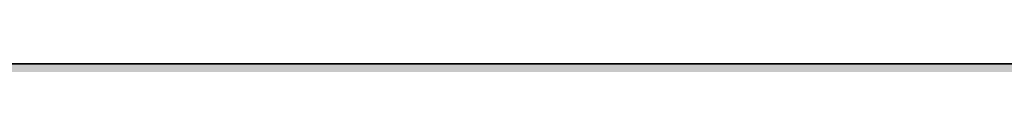
# Model space of a CAD drawing. Units: inches. Extents: x 2091 to 2899, y 967 to 2217.
# Tile 70 of 256: x 2213.35 to 2214.757, y 1099.919 to 1099.919. Entities that reach past the tile are written whole.
import ezdxf

# ---------------------------------------------------------------- set-up
doc = ezdxf.new("R2010")
doc.units = ezdxf.units.IN
doc.layers.add('A-WALL-PATT', color=141, linetype='Continuous', lineweight=13, true_color=0xadddf7)
doc.layers.add('L-SITE-WALL', color=7, linetype='Continuous', lineweight=35)

msp = doc.modelspace()

# ---------------------------------------------------------------- hatches: boundary and pattern name
at = {"layer": 'A-WALL-PATT'}
h = msp.add_hatch(color=256, dxfattribs=at)
h.dxf.hatch_style = 1
h.paths.add_polyline_path([(2212.1436, 1941.4191), (2387.6436, 1941.4191), (2387.6436, 1824.4191), (2392.1436, 1824.4191), (2392.1436, 1941.4191), (2609.6436, 1941.4191), (2609.6436, 1825.9191), (2614.1436, 1825.9191), (2614.1436, 1941.4191), (2794.1436, 1941.4191), (2794.1436, 1928.7622), (2803.1436, 1928.7622), (2803.1436, 2050.9191), (2203.1436, 2050.9191), (2203.1436, 1900.7579), (2212.1436, 1900.7579)])
h.paths.add_polyline_path([(2212.1436, 1945.9191), (2212.1436, 2041.9191), (2794.1436, 2041.9191), (2794.1436, 1945.9191), (2402.2482, 1945.9191), (2401.1024, 1945.7758), (2398.7024, 1945.7758)], flags=16)
h.paths.add_polyline_path([(2230.2299, 1948.0628), (2227.3499, 1949.5028), (2225.9099, 1951.9028), (2223.9899, 1952.8628), (2223.0299, 1955.2628), (2222.0699, 1959.5828), (2222.0699, 1963.4228), (2223.0299, 1965.6628), (2223.9899, 1965.3428), (2225.5859, 1963.8607), (2226.9115, 1964.9573), (2226.9489, 1965.9388), (2227.7783, 1966.9521), (2228.1999, 1968.8787), (2230.7099, 1964.8628), (2233.5899, 1966.3028), (2233.6073, 1966.3319), (2233.7727, 1964.9382), (2234.6338, 1963.6765), (2235.0299, 1963.9028), (2236.282, 1965.5724), (2235.9899, 1962.9428), (2237.9545, 1957.54), (2238.3899, 1957.9028), (2239.2159, 1960.3058), (2238.6546, 1966.385), (2238.6928, 1966.4381), (2238.8406, 1967.4997), (2238.7803, 1967.6875), (2238.8805, 1967.7868), (2238.6669, 1966.2518), (2239.2159, 1960.3058), (2238.3899, 1957.9028), (2236.9499, 1956.7028), (2234.5499, 1949.9828)], flags=0)
h.paths.add_polyline_path([(2278.012, 1948.0628), (2276.4964, 1947.8733), (2275.8498, 1947.6886), (2274.652, 1947.1028)], flags=0)
h.paths.add_polyline_path([(2269.852, 1955.7428), (2268.2762, 1956.6293), (2270.8673, 1956.3484), (2269.372, 1958.1428), (2268.715, 1959.1923), (2270.5698, 1958.7286), (2268.5807, 1961.9061), (2270.812, 1960.8919), (2270.812, 1963.4228), (2271.3933, 1964.7793), (2270.2918, 1966.1562), (2271.772, 1965.6628), (2272.1414, 1966.5248), (2273.9298, 1965.9286), (2275.6304, 1968.0543), (2276.3319, 1966.7219), (2276.5204, 1966.9521), (2276.942, 1968.8787), (2277.7343, 1967.6111), (2278.1399, 1969.4645), (2279.6591, 1967.0337), (2280.412, 1966.7828), (2280.9493, 1967.5888), (2281.6098, 1967.3686), (2282.1333, 1968.1538), (2282.3492, 1966.3334), (2282.3498, 1966.3326), (2283.4076, 1968.0954), (2283.7126, 1965.524), (2284.3202, 1964.6338), (2284.5118, 1964.8892), (2284.235, 1965.7048), (2284.5005, 1967.319), (2284.9079, 1965.4174), (2285.3963, 1966.0686), (2285.4328, 1966.2906), (2285.4733, 1966.1713), (2286.3539, 1967.3454), (2286.222, 1966.1582), (2287.6635, 1968.0802), (2287.714, 1968.4428), (2288.4816, 1969.0167), (2288.574, 1968.7289), (2288.9175, 1969.069), (2288.6068, 1966.8376), (2288.9287, 1963.3513), (2288.935, 1963.3568), (2288.9297, 1963.3404), (2289.0153, 1962.4139), (2290.1112, 1963.8751), (2290.1328, 1963.9426), (2290.2177, 1964.0171), (2290.1112, 1963.8751), (2289.1558, 1960.8916), (2288.594, 1959.2572), (2288.572, 1959.1028), (2289.532, 1960.5428), (2290.012, 1962.4628), (2290.1918, 1962.6427), (2289.7698, 1959.6886), (2286.8898, 1957.2886), (2284.4898, 1950.5686), (2283.3147, 1950.0463), (2283.292, 1949.9828), (2280.2901, 1948.6486), (2281.1298, 1948.6486), (2282.5698, 1948.1686), (2283.2047, 1948.0628), (2278.972, 1948.0628), (2276.092, 1949.5028), (2274.652, 1951.9028), (2272.732, 1952.8628)], flags=0)
h.paths.add_polyline_path([(2271.1589, 1958.0218), (2272.9698, 1955.8486), (2272.0098, 1960.1686), (2272.0098, 1964.0086), (2272.6244, 1965.4427), (2274.328, 1963.8607), (2275.6536, 1964.9573), (2275.6377, 1964.5391), (2277.4122, 1966.0069), (2277.033, 1965.1568), (2276.8299, 1964.9756), (2276.766, 1963.295), (2277.4496, 1962.6602), (2279.452, 1964.8628), (2282.332, 1966.3028), (2283.5298, 1966.8886), (2283.2945, 1966.7709), (2283.913, 1963.8847), (2284.8992, 1964.4483), (2284.732, 1962.9428), (2286.6966, 1957.54), (2287.132, 1957.9028), (2287.5419, 1959.0954), (2287.7794, 1958.4423), (2285.6827, 1956.6951), (2285.8765, 1959.7953), (2284.732, 1962.9428), (2284.8992, 1964.4483), (2283.913, 1963.8847), (2284.2238, 1962.4341), (2283.4244, 1963.6055), (2281.6098, 1962.5686), (2281.1298, 1960.1686), (2282.0898, 1956.3286), (2283.0498, 1952.9686), (2282.5698, 1950.5686), (2280.1698, 1948.6486), (2279.8833, 1948.7919), (2278.972, 1948.0628), (2278.972, 1949.0228), (2278.6723, 1949.3974), (2277.2898, 1950.0886), (2275.8498, 1952.4886), (2273.9298, 1953.4486), (2272.4898, 1954.8886), (2271.9216, 1954.8886), (2271.772, 1955.2628)], flags=0)
h.paths.add_polyline_path([(2311.9941, 1955.7428), (2312.0627, 1955.6742), (2312.0551, 1955.7085)], flags=0)
h.paths.add_polyline_path([(2331.9561, 1963.9518), (2333.3961, 1965.3918), (2331.0771, 1963.3568), (2330.9986, 1963.1115)], flags=0)
h.paths.add_polyline_path([(2310.5541, 1954.3028), (2307.0398, 1956.2799), (2310.7629, 1955.8763), (2312.4741, 1953.8228), (2313.4341, 1951.4228), (2315.3541, 1950.4628), (2316.7941, 1948.0628), (2317.4661, 1947.7268), (2319.3687, 1947.9646), (2317.7541, 1949.9828), (2317.5695, 1950.6105), (2316.7941, 1951.9028), (2314.8741, 1952.8628), (2313.9141, 1955.2628), (2311.5141, 1958.1428), (2309.3755, 1961.5592), (2311.5141, 1960.3371), (2311.5141, 1961.9828), (2310.6047, 1963.1196), (2311.7266, 1962.4785), (2312.4183, 1964.0926), (2312.256, 1964.2955), (2313.1941, 1963.9828), (2313.9141, 1965.6628), (2314.6468, 1965.4186), (2315.3541, 1966.3028), (2316.7941, 1967.7428), (2316.1574, 1966.9469), (2317.0341, 1965.2819), (2317.2226, 1965.5121), (2317.777, 1968.0458), (2318.4741, 1966.7219), (2318.6626, 1966.9521), (2319.0842, 1968.8787), (2321.207, 1965.4821), (2322.1614, 1966.9137), (2322.5541, 1966.7828), (2322.786, 1967.1306), (2322.8816, 1966.3243), (2323.312, 1965.7217), (2323.6513, 1965.8914), (2324.3965, 1967.1334), (2324.6569, 1964.9382), (2324.972, 1964.4766), (2325.3873, 1967.0015), (2325.9408, 1964.4183), (2327.2289, 1966.1358), (2327.1663, 1965.5724), (2328.0591, 1966.7628), (2328.2246, 1966.2475), (2329.668, 1967.6769), (2329.6646, 1967.6875), (2329.7648, 1967.7868), (2329.5511, 1966.2518), (2330.1001, 1960.3058), (2329.3328, 1958.0735), (2329.3131, 1957.9352), (2329.6341, 1958.2028), (2330.2341, 1959.1028), (2330.7141, 1961.0228), (2331.0341, 1961.3428), (2330.7141, 1959.1028), (2329.6341, 1958.2028), (2329.2741, 1957.6628), (2327.7121, 1956.3611), (2325.4341, 1949.9828), (2324.3338, 1949.4937), (2323.9941, 1948.5428), (2319.6741, 1946.6228), (2316.7941, 1948.0628), (2315.3541, 1950.4628), (2313.4341, 1951.4228)], flags=0)
h.paths.add_polyline_path([(2321.3357, 1947.952), (2321.1141, 1948.0628), (2321.1141, 1949.0228), (2319.1941, 1951.4228), (2316.7941, 1959.5828), (2316.6632, 1959.5828), (2315.3541, 1958.1428), (2314.3941, 1958.1428), (2313.1483, 1958.7091), (2312.9541, 1959.5828), (2312.9541, 1960.8919), (2315.8341, 1959.5828), (2316.6632, 1959.5828), (2317.3147, 1960.2994), (2315.0302, 1962.4207), (2316.3558, 1963.5173), (2316.3723, 1963.9516), (2316.4702, 1963.8607), (2317.7958, 1964.9573), (2317.7552, 1963.8897), (2319.1751, 1965.1568), (2319.4984, 1965.8814), (2321.1141, 1965.3428), (2323.2359, 1962.3724), (2325.6863, 1963.7726), (2325.5428, 1962.4806), (2325.1988, 1963.494), (2324.4785, 1963.0824), (2324.926, 1960.9941), (2324.0781, 1962.2365), (2322.4148, 1961.286), (2322.0741, 1959.5828), (2323.0341, 1955.7428), (2323.9941, 1952.3828), (2323.5141, 1949.9828), (2322.1427, 1948.8856), (2322.0741, 1948.5428)], flags=0)
h.paths.add_polyline_path([(2320.2075, 1963.3375), (2320.1541, 1963.4228), (2320.3941, 1963.5428)], flags=0)
h.paths.add_polyline_path([(2353.8505, 1965.8105), (2354.0305, 1965.7505), (2354.3305, 1966.4505), (2354.3305, 1966.9305)], flags=0)
h.paths.add_polyline_path([(2359.0206, 1969.0264), (2359.0984, 1968.9019), (2359.2335, 1969.5195), (2359.2335, 1969.9995)], flags=0)
h.paths.add_polyline_path([(2358.2567, 1966.6817), (2357.9836, 1966.348), (2358.2113, 1966.1462), (2358.4105, 1966.3896)], flags=0)
h.paths.add_polyline_path([(2357.7685, 1966.0588), (2357.7322, 1965.105), (2357.751, 1965.1206), (2357.7695, 1965.6065), (2357.7695, 1966.0578)], flags=0)
h.paths.add_polyline_path([(2359.1115, 1965.3045), (2359.1115, 1964.8245), (2359.8445, 1966.4675), (2359.8445, 1966.9475)], flags=0)
h.paths.add_polyline_path([(2360.2237, 1966.6214), (2360.6985, 1969.3625), (2360.6985, 1969.8425), (2360.2105, 1967.0255), (2360.2105, 1966.6425)], flags=0)
h.paths.add_polyline_path([(2363.4505, 1967.8905), (2363.4505, 1968.3705), (2362.4905, 1966.9305), (2362.656, 1966.6988)], flags=0)
h.paths.add_polyline_path([(2364.4755, 1966.0788), (2365.8505, 1968.3705), (2365.8505, 1968.8505), (2364.428, 1966.4796)], flags=0)
h.paths.add_polyline_path([(2366.3135, 1965.8525), (2366.3667, 1965.6958), (2366.8025, 1968.3455), (2366.8025, 1968.8255)], flags=0)
h.paths.add_polyline_path([(2367.1653, 1965.8035), (2367.2905, 1966.9305), (2367.2905, 1967.4105), (2367.1027, 1965.7201)], flags=0)
h.paths.add_polyline_path([(2370.0365, 1959.9735), (2371.0135, 1963.0245), (2371.0135, 1963.5045), (2370.0365, 1960.4535)], flags=0)
h.paths.add_polyline_path([(2371.6105, 1960.2105), (2372.5705, 1961.6505), (2372.5705, 1962.1305), (2371.8025, 1960.9785)], flags=0)
h.paths.add_polyline_path([(2350.8737, 1956.0051), (2351.9305, 1955.8905), (2354.4905, 1953.3305), (2353.8505, 1954.9305), (2351.4505, 1957.8105), (2347.9355, 1963.4255), (2347.9355, 1963.9055), (2351.4505, 1958.2905), (2353.7051, 1955.585), (2352.8905, 1959.2505), (2352.8905, 1959.7305), (2352.8905, 1961.9248), (2356.7305, 1959.7305), (2358.4545, 1961.6268), (2354.8105, 1965.0105), (2355.0309, 1965.2859), (2358.6911, 1961.8871), (2361.5305, 1965.0105), (2364.3765, 1966.4335), (2364.5244, 1965.1869), (2365.4545, 1963.8242), (2365.8811, 1964.068), (2365.3705, 1966.4505), (2365.3705, 1966.9305), (2366.8105, 1960.2105), (2366.8105, 1959.7305), (2366.3887, 1952.9814), (2367.7705, 1956.8505), (2368.6412, 1957.5761), (2366.8105, 1962.6105), (2366.8105, 1963.0905), (2368.7752, 1957.6877), (2369.2105, 1958.0505), (2370.0016, 1960.3519), (2369.4752, 1966.0527), (2369.5135, 1966.1058), (2369.5142, 1966.1109), (2369.4752, 1966.5327), (2369.5135, 1966.5858), (2369.6146, 1967.3126), (2369.1825, 1968.6585), (2369.1825, 1969.1385), (2369.601, 1967.8352), (2369.7012, 1967.9345), (2369.7179, 1968.0547), (2370.1452, 1968.3741), (2369.7787, 1968.0112), (2369.7012, 1967.4545), (2370.4682, 1968.214), (2369.6749, 1967.2658), (2369.5142, 1966.1109), (2370.0365, 1960.4535), (2370.0365, 1959.9735), (2369.4418, 1958.2432), (2370.6505, 1959.2505), (2371.0458, 1962.0176), (2371.1305, 1962.1305), (2370.6505, 1958.7705), (2367.7705, 1956.3705), (2365.3705, 1949.6505), (2362.0791, 1948.1876), (2363.4505, 1947.7305), (2361.0505, 1947.7305), (2360.0905, 1947.7305), (2357.1039, 1947.3572), (2360.0905, 1948.2105), (2358.1705, 1949.1705), (2356.7305, 1951.5705), (2354.8105, 1952.5305), (2351.9305, 1955.4105)], flags=0)
h.paths.add_polyline_path([(2361.0505, 1948.6905), (2359.1305, 1951.0905), (2356.7305, 1959.2505), (2355.7705, 1959.2505), (2352.8905, 1960.5596), (2352.8905, 1961.4448), (2355.8905, 1959.7305), (2356.7305, 1959.7305), (2356.8372, 1959.3678), (2361.5305, 1964.5305), (2363.2484, 1965.3894), (2364.9253, 1963.0418), (2362.4905, 1961.6505), (2362.0639, 1959.5172), (2362.9705, 1955.8905), (2363.9305, 1952.5305), (2363.9305, 1952.0505), (2363.4505, 1949.6505), (2361.0505, 1947.7305)], flags=0)
h.paths.add_polyline_path([(2359.1305, 1951.5705), (2359.2905, 1951.3705), (2361.0505, 1954.4505), (2361.0505, 1954.9305)], flags=0)
h.paths.add_polyline_path([(2357.2195, 1966.5455), (2356.7925, 1968.8145), (2356.7925, 1969.2945), (2357.2195, 1967.0255)], flags=0)
h.paths.add_polyline_path([(2361.0505, 1954.4505), (2361.5305, 1958.7705), (2361.5305, 1959.2505), (2361.0505, 1954.9305)], flags=0)
h.paths.add_polyline_path([(2402.5483, 1948.4861), (2402.3024, 1948.4158), (2402.5904, 1948.4158)], flags=0)
h.paths.add_polyline_path([(2394.1424, 1956.0958), (2395.6851, 1954.5532), (2396.7205, 1953.9707), (2396.0624, 1955.6158), (2395.2414, 1956.6011), (2395.8789, 1956.4417), (2395.1024, 1959.9358), (2395.1024, 1963.7758), (2396.0624, 1966.0158), (2397.0224, 1965.6958), (2398.6185, 1964.2138), (2399.9441, 1965.3103), (2399.9814, 1966.2918), (2400.8109, 1967.3052), (2401.2325, 1969.2317), (2403.5379, 1965.543), (2403.942, 1967.3893), (2404.7024, 1967.1358), (2405.4603, 1966.0748), (2406.6224, 1966.6558), (2406.6399, 1966.6849), (2406.8052, 1965.2912), (2406.9257, 1965.1147), (2407.3424, 1964.9758), (2407.8743, 1965.7737), (2408.1691, 1964.3981), (2409.3146, 1965.9254), (2409.2175, 1965.0511), (2409.4452, 1963.1312), (2410.3064, 1961.8695), (2410.7024, 1962.0958), (2411.4423, 1963.0823), (2411.1654, 1963.8978), (2411.6164, 1966.6398), (2411.7254, 1966.7911), (2411.8732, 1967.8527), (2411.8129, 1968.0405), (2411.9131, 1968.1398), (2411.6994, 1966.6048), (2412.2484, 1960.6588), (2413.2254, 1963.7098), (2414.3779, 1964.7212), (2414.5132, 1965.6927), (2414.4529, 1965.8805), (2414.5531, 1965.9798), (2414.3779, 1964.7212), (2414.5198, 1964.8457), (2414.3654, 1964.6311), (2414.3394, 1964.4448), (2414.8884, 1958.4988), (2414.0624, 1956.0958), (2412.6224, 1954.8958), (2410.1714, 1948.0329), (2410.0167, 1948.0844), (2405.9024, 1946.2558), (2405.9024, 1947.2158), (2405.2043, 1948.0886), (2404.2224, 1948.4158), (2403.2624, 1948.4158), (2400.3824, 1949.8558), (2399.6624, 1951.0558), (2397.9824, 1952.7358), (2397.0224, 1953.2158), (2395.6851, 1954.5532), (2392.6568, 1956.2569)], flags=0)
h.paths.add_polyline_path([(2409.0857, 1964.4074), (2409.1304, 1964.2757), (2409.2624, 1964.4958)], flags=0)
h.paths.add_polyline_path([(2397.7424, 1961.6158), (2398.7024, 1963.8558), (2399.6624, 1963.5358), (2401.4266, 1965.741), (2401.7914, 1966.5588), (2402.0714, 1965.0708), (2402.8355, 1964.3934), (2403.2624, 1964.9149), (2403.3381, 1964.7711), (2402.6155, 1963.9762), (2402.4986, 1960.9022), (2403.543, 1959.9325), (2404.4132, 1960.8897), (2404.7024, 1962.3358), (2407.9163, 1964.1724), (2409.5202, 1961.9269), (2410.9871, 1957.893), (2411.4224, 1958.2558), (2412.048, 1960.0756), (2412.4103, 1959.0791), (2411.6756, 1958.4668), (2411.6624, 1958.2558), (2411.6261, 1958.4255), (2409.9824, 1957.0558), (2407.5824, 1950.3358), (2403.2624, 1948.4158), (2403.2624, 1949.3758), (2401.3424, 1951.7758), (2399.4165, 1958.324), (2397.7424, 1959.0849), (2397.7424, 1959.9701), (2397.1024, 1960.3358), (2397.7424, 1960.0449)], flags=0)
h.paths.add_polyline_path([(2405.9024, 1952.9758), (2405.9504, 1953.4078), (2406.0167, 1953.1758)], flags=0)
h.paths.add_polyline_path([(2449.8178, 1967.114), (2449.7523, 1967.1358), (2449.7937, 1967.0779)], flags=0)
h.paths.add_polyline_path([(2451.6977, 1966.6181), (2451.7409, 1966.6901), (2451.6921, 1966.6657)], flags=0)
h.paths.add_polyline_path([(2454.3436, 1965.7376), (2455.7523, 1967.6158), (2455.9923, 1968.0958), (2454.3645, 1965.9254)], flags=0)
h.paths.add_polyline_path([(2457.5473, 1968.8638), (2457.7873, 1969.3438), (2457.0543, 1968.7958), (2457.0076, 1968.4603)], flags=0)
h.paths.add_polyline_path([(2456.9218, 1967.8567), (2456.8022, 1968.229), (2456.723, 1967.6598)], flags=0)
h.paths.add_polyline_path([(2457.3023, 1967.3768), (2457.5423, 1967.8568), (2456.8103, 1966.8398), (2456.7405, 1966.7002), (2456.749, 1966.6081)], flags=0)
h.paths.add_polyline_path([(2458.2753, 1963.7098), (2458.1553, 1963.3352), (2460.3543, 1965.2648), (2460.5943, 1965.7448)], flags=0)
h.paths.add_polyline_path([(2458.3923, 1962.8158), (2458.3641, 1962.6182), (2459.5923, 1964.2558), (2459.8323, 1964.7358)], flags=0)
h.paths.add_polyline_path([(2459.3523, 1962.8158), (2459.2723, 1962.4958), (2460.0723, 1963.2958), (2460.3123, 1963.7758)], flags=0)
h.paths.add_polyline_path([(2458.6803, 1960.6078), (2458.6323, 1960.4158), (2459.5923, 1961.8558), (2459.8323, 1962.3358)], flags=0)
h.paths.add_polyline_path([(2437.8382, 1956.2427), (2439.1923, 1956.0958), (2441.3523, 1953.9358), (2440.8723, 1955.1358), (2438.4723, 1958.0158), (2438.0716, 1958.656), (2438.7123, 1958.4958), (2440.6396, 1956.1831), (2439.9123, 1959.4558), (2439.9123, 1963.2958), (2441.3523, 1966.6558), (2441.5923, 1967.1358), (2441.1123, 1966.0158), (2442.0723, 1965.6958), (2443.989, 1968.0917), (2444.2413, 1966.7508), (2444.9168, 1966.1519), (2445.6766, 1967.0801), (2446.2553, 1969.7248), (2446.4953, 1970.2048), (2446.2824, 1969.2317), (2447.3627, 1967.5033), (2447.7203, 1969.5678), (2447.9603, 1970.0478), (2447.4855, 1967.3068), (2448.7923, 1965.2158), (2448.4723, 1964.8638), (2448.5523, 1964.7358), (2451.4521, 1966.1857), (2451.6151, 1964.8112), (2452.3079, 1963.7962), (2453.2345, 1964.3257), (2454.0723, 1960.4158), (2453.6287, 1953.3177), (2454.7923, 1956.5758), (2455.0323, 1957.0558), (2455.7188, 1957.6279), (2453.8323, 1962.8158), (2453.941, 1963.7936), (2453.3353, 1965.5778), (2453.8243, 1968.5508), (2454.0643, 1969.0308), (2453.5753, 1966.0578), (2454.0403, 1964.6879), (2453.8323, 1962.8158), (2455.7188, 1957.6279), (2456.3672, 1958.1682), (2457.0583, 1960.1788), (2457.2983, 1960.6588), (2456.4723, 1958.2558), (2457.7177, 1959.2937), (2457.6723, 1958.9758), (2454.89, 1956.6572), (2453.6141, 1953.0849), (2453.5923, 1952.7358), (2453.3523, 1952.2558), (2453.3596, 1952.3722), (2452.6323, 1950.3358), (2452.3923, 1949.8558), (2449.2038, 1948.4387), (2450.7123, 1947.9358), (2448.0723, 1947.9358), (2447.1123, 1947.9358), (2444.5523, 1947.6158), (2447.1996, 1948.3722), (2445.1923, 1949.3758), (2443.7523, 1951.7758), (2441.8323, 1952.7358), (2438.9523, 1955.6158)], flags=0)
h.paths.add_polyline_path([(2443.9923, 1959.9358), (2444.0403, 1959.7726), (2444.1216, 1959.862)], flags=0)
h.paths.add_polyline_path([(2442.9123, 1959.9358), (2443.0323, 1959.9358), (2442.4457, 1960.2025)], flags=0)
h.paths.add_polyline_path([(2444.9829, 1965.0197), (2445.2793, 1965.2648), (2445.5193, 1965.7448), (2444.994, 1965.3103)], flags=0)
h.paths.add_polyline_path([(2446.1333, 1965.0298), (2446.3304, 1965.4715), (2444.9703, 1964.2578), (2444.7303, 1963.7778)], flags=0)
h.paths.add_polyline_path([(2442.7923, 1959.4558), (2443.7523, 1959.4558), (2446.1523, 1951.2958), (2446.4123, 1951.7508), (2446.3923, 1951.7758), (2448.0806, 1954.7303), (2448.5523, 1958.9758), (2441.8323, 1965.2158), (2442.1549, 1965.6191), (2448.7923, 1959.4558), (2448.3123, 1955.1358), (2448.0723, 1954.6558), (2446.4123, 1951.7508), (2448.3123, 1949.3758), (2448.3123, 1948.4158), (2450.5409, 1950.1987), (2450.9523, 1952.2558), (2449.9923, 1955.6158), (2449.0323, 1959.4558), (2449.5123, 1961.8558), (2449.7523, 1962.3358), (2449.6749, 1961.9487), (2452.9945, 1963.8457), (2453.0644, 1963.5194), (2452.8846, 1963.7829), (2449.6749, 1961.9487), (2449.2723, 1959.9358), (2450.2323, 1956.0958), (2451.1923, 1952.7358), (2450.7123, 1950.3358), (2450.4723, 1949.8558), (2448.0723, 1947.9358), (2448.0723, 1948.5358), (2445.4323, 1949.8558), (2443.9923, 1952.2558), (2442.0723, 1953.2158), (2441.1123, 1955.6158), (2440.1523, 1959.9358), (2440.1523, 1960.6558)], flags=0)
h.paths.add_polyline_path([(2456.6923, 1966.9858), (2457.6083, 1968.0808), (2457.8483, 1968.5608), (2456.9323, 1967.4658)], flags=0)
h.paths.add_polyline_path([(2489.8966, 1966.5802), (2489.9429, 1966.1893), (2490.7475, 1967.5302), (2491.3191, 1968.9512)], flags=0)
h.paths.add_polyline_path([(2473.5625, 1956.4071), (2477.14, 1956.0193), (2476.9553, 1956.2408), (2475.108, 1957.2801), (2476.3475, 1956.9702), (2475.1869, 1958.8242), (2476.9191, 1958.3912), (2475.4116, 1960.7993), (2477.7875, 1959.7193), (2477.7875, 1962.2502), (2477.6374, 1962.4379), (2477.8226, 1962.3321), (2478.3591, 1963.5841), (2478.3591, 1963.6712), (2477.3243, 1964.9646), (2478.7148, 1964.5011), (2479.3191, 1965.9112), (2480.2791, 1965.5912), (2481.784, 1967.4722), (2482.1165, 1965.7052), (2482.8806, 1965.0278), (2483.2093, 1965.4294), (2483.2202, 1965.7151), (2483.0759, 1965.989), (2483.7118, 1966.7658), (2484.1305, 1968.6792), (2484.7021, 1970.1002), (2484.4892, 1969.1271), (2486.5029, 1965.9051), (2487.3875, 1965.6102), (2488.1534, 1966.7591), (2488.717, 1965.9701), (2489.2001, 1966.2116), (2489.3307, 1965.111), (2490.3939, 1963.6225), (2490.6608, 1963.775), (2490.4939, 1964.5536), (2490.9231, 1963.9248), (2491.3191, 1964.1512), (2491.3334, 1964.1702), (2491.2105, 1964.5322), (2491.2818, 1964.9655), (2491.4258, 1964.2934), (2494.0765, 1967.8276), (2494.4979, 1966.5149), (2494.5982, 1966.6142), (2494.6895, 1967.2702), (2495.1067, 1967.5822), (2495.1298, 1967.7481), (2495.0696, 1967.9359), (2495.1698, 1968.0351), (2495.0318, 1967.0436), (2495.7538, 1967.7587), (2494.9821, 1966.6864), (2494.9561, 1966.5002), (2495.479, 1960.8369), (2495.9105, 1962.1842), (2496.4821, 1963.6052), (2496.0727, 1962.3266), (2496.7689, 1962.9375), (2496.5991, 1962.7112), (2496.1191, 1959.3512), (2496.7329, 1960.2718), (2496.9875, 1961.2902), (2497.5591, 1962.7112), (2497.0791, 1960.7912), (2496.5075, 1959.3702), (2495.5475, 1957.9302), (2492.7588, 1955.6064), (2490.8391, 1950.2312), (2490.2675, 1948.8102), (2485.9475, 1946.8902), (2483.0675, 1948.3302), (2481.6275, 1950.7302), (2479.7075, 1951.6902), (2476.8275, 1954.5702)], flags=0)
h.paths.add_polyline_path([(2485.577, 1948.3134), (2485.5591, 1948.3112), (2485.5788, 1948.3112)], flags=0)
h.paths.add_polyline_path([(2478.6451, 1954.5512), (2478.109, 1956.9633), (2479.3191, 1955.5112), (2480.2791, 1953.1112), (2482.1991, 1952.1512), (2483.6391, 1949.7512), (2486.5191, 1948.3112), (2486.5191, 1949.2712), (2484.7393, 1951.4959), (2484.0275, 1950.2502), (2481.6275, 1958.4102), (2482.3751, 1959.2327), (2482.1991, 1959.8312), (2483.1976, 1960.9295), (2479.7075, 1964.1702), (2480.6034, 1965.2901), (2481.8752, 1964.1091), (2482.6664, 1964.7636), (2482.6154, 1963.4218), (2482.9892, 1963.0747), (2484.0085, 1963.9842), (2484.6836, 1965.4975), (2484.5801, 1965.4052), (2485.3573, 1967.1471), (2485.1206, 1965.7812), (2486.4275, 1963.6902), (2488.1454, 1964.5492), (2489.8223, 1962.2016), (2490.7475, 1962.7302), (2491.9997, 1964.3998), (2492.076, 1965.0873), (2492.2129, 1964.6841), (2492.4854, 1965.0474), (2492.2791, 1963.1912), (2494.2438, 1957.7884), (2494.5625, 1958.054), (2494.9335, 1959.1332), (2495.5051, 1960.5542), (2494.6791, 1958.1512), (2494.1075, 1956.7302), (2494.5625, 1958.054), (2493.4085, 1957.0923), (2491.7075, 1961.7702), (2491.9997, 1964.3998), (2490.7475, 1962.7302), (2487.712, 1960.9957), (2487.4791, 1959.8312), (2488.4391, 1955.9912), (2489.3991, 1952.6312), (2488.9191, 1950.2312), (2488.5769, 1949.9574), (2488.3475, 1948.8102), (2487.6517, 1948.2536), (2487.4791, 1948.3112), (2486.5191, 1948.3112), (2483.6391, 1949.7512), (2482.1991, 1952.1512), (2480.2791, 1953.1112), (2478.8391, 1954.5512)], flags=0)
h.paths.add_polyline_path([(2526.6483, 1966.9875), (2526.5173, 1967.0312), (2526.6001, 1966.9153)], flags=0)
h.paths.add_polyline_path([(2528.4706, 1966.4467), (2528.5745, 1966.6197), (2528.4571, 1966.561)], flags=0)
h.paths.add_polyline_path([(2534.1333, 1967.4962), (2534.1567, 1967.5428), (2534.0598, 1967.4083)], flags=0)
h.paths.add_polyline_path([(2536.1619, 1964.0506), (2535.1573, 1962.7112), (2535.1009, 1962.3159), (2536.1173, 1963.6712), (2536.4205, 1964.2775)], flags=0)
h.paths.add_polyline_path([(2535.1573, 1959.8312), (2536.1173, 1961.2712), (2536.5973, 1962.2312), (2535.2533, 1960.2152)], flags=0)
h.paths.add_polyline_path([(2513.249, 1956.2848), (2516.2212, 1955.9626), (2514.9973, 1957.4312), (2514.1958, 1958.7115), (2515.4773, 1958.3912), (2516.9319, 1956.6457), (2516.4373, 1958.8712), (2516.4373, 1962.7112), (2516.8727, 1963.727), (2515.3464, 1965.6348), (2517.3973, 1964.9512), (2517.8773, 1966.0712), (2518.3573, 1967.0312), (2517.8773, 1965.9112), (2518.8373, 1965.5912), (2520.4866, 1967.6527), (2520.7663, 1966.1662), (2521.5304, 1965.4887), (2521.7814, 1965.7954), (2521.8009, 1966.3073), (2521.4778, 1966.9209), (2521.2463, 1967.1262), (2521.1777, 1967.4909), (2521.4778, 1966.9209), (2522.0104, 1966.4487), (2522.2574, 1966.7504), (2522.7803, 1969.1402), (2523.2603, 1970.1002), (2523.0474, 1969.1271), (2524.6731, 1966.5259), (2526.0373, 1966.0712), (2526.7952, 1965.0101), (2527.9771, 1965.601), (2528.1401, 1964.2266), (2528.6646, 1963.4582), (2529.3886, 1963.8719), (2529.3297, 1964.147), (2529.4813, 1963.9248), (2529.8773, 1964.1512), (2529.984, 1964.2934), (2529.7891, 1965.2032), (2530.0624, 1964.3979), (2532.8025, 1968.0513), (2533.1478, 1966.9759), (2533.248, 1967.0751), (2533.3393, 1967.7312), (2533.6728, 1967.9805), (2533.728, 1968.0351), (2533.5143, 1966.5002), (2534.0247, 1960.9725), (2534.5603, 1962.6452), (2535.0403, 1963.6052), (2534.0633, 1960.5542), (2533.2373, 1958.1512), (2534.2882, 1959.0268), (2534.1973, 1958.3912), (2531.5126, 1956.1539), (2529.3973, 1950.2312), (2528.9173, 1949.2712), (2526.4488, 1948.174), (2527.4773, 1947.8312), (2530.3573, 1947.3512), (2524.5973, 1947.3512), (2521.7173, 1948.7912), (2520.2773, 1951.1912), (2518.3573, 1952.1512), (2515.4773, 1955.0312)], flags=0)
h.paths.add_polyline_path([(2523.9348, 1967.1903), (2523.6195, 1966.4837), (2523.7705, 1966.2421)], flags=0)
h.paths.add_polyline_path([(2518.8373, 1953.1112), (2517.8773, 1955.5112), (2516.885, 1959.9768), (2516.9173, 1959.9621), (2516.9173, 1962.0254), (2520.7573, 1959.8312), (2522.0249, 1961.2255), (2518.3573, 1964.6312), (2519.0026, 1965.4377), (2520.4334, 1964.1091), (2521.3011, 1964.8269), (2521.2452, 1963.3553), (2525.6383, 1959.276), (2526.0373, 1961.2712), (2529.3973, 1963.1912), (2530.6495, 1964.8607), (2530.6647, 1964.9976), (2530.692, 1964.9173), (2531.0878, 1965.4451), (2530.946, 1964.1689), (2530.692, 1964.9173), (2529.3973, 1963.1912), (2526.3625, 1961.457), (2526.0373, 1959.8312), (2526.9973, 1955.9912), (2527.9573, 1952.6312), (2527.4773, 1950.2312), (2527.1345, 1949.9569), (2526.9739, 1949.1541), (2526.6973, 1949.0312), (2524.5973, 1947.3512), (2524.5973, 1948.3112), (2524.2773, 1948.7112), (2522.1973, 1949.7512), (2520.7573, 1952.1512)], flags=0)
h.paths.add_polyline_path([(2520.2773, 1958.8712), (2520.8533, 1959.5048), (2523.1573, 1951.6712), (2524.6139, 1954.2201), (2524.5973, 1954.0712), (2522.6773, 1950.7112)], flags=0)
h.paths.add_polyline_path([(2559.3709, 1966.3112), (2559.3984, 1966.3249), (2559.4019, 1966.3453)], flags=0)
h.paths.add_polyline_path([(2549.7709, 1957.1912), (2552.6509, 1954.3112), (2552.134, 1955.6035), (2550.6109, 1957.4312), (2547.0959, 1963.0462), (2545.7759, 1965.2062), (2549.2909, 1959.5912), (2551.6909, 1956.7112), (2550.7929, 1960.7521), (2550.7309, 1960.7803), (2550.7309, 1964.8712), (2551.6909, 1967.1112), (2552.6509, 1966.7912), (2554.247, 1965.3091), (2555.0343, 1965.9603), (2555.5817, 1966.6446), (2555.6099, 1967.3872), (2556.4394, 1968.4005), (2556.861, 1970.3271), (2559.3709, 1966.3112), (2560.6909, 1964.1512), (2562.4088, 1965.0101), (2561.6509, 1966.0712), (2560.3309, 1968.2312), (2561.7585, 1966.2325), (2562.3472, 1967.1156), (2562.4337, 1966.3866), (2563.1278, 1965.3696), (2563.5709, 1965.5912), (2563.5884, 1965.6202), (2563.3625, 1967.5235), (2563.7225, 1965.8438), (2565.06, 1968.073), (2564.7329, 1965.1287), (2565.1176, 1963.3334), (2567.4446, 1966.4361), (2567.3156, 1967.8333), (2567.3538, 1967.8864), (2567.5016, 1968.9481), (2567.4413, 1969.1359), (2567.5416, 1969.2351), (2567.3279, 1967.7002), (2567.8769, 1961.7542), (2568.7467, 1964.4703), (2568.6356, 1965.6733), (2568.6738, 1965.7264), (2568.8216, 1966.7881), (2568.7613, 1966.9759), (2568.8616, 1967.0751), (2568.6479, 1965.5402), (2568.7261, 1964.693), (2568.8539, 1964.8052), (2568.7467, 1964.4703), (2568.8172, 1963.7063), (2568.9709, 1963.9112), (2568.8661, 1963.1773), (2569.1969, 1959.5942), (2568.3709, 1957.1912), (2566.9309, 1955.9912), (2564.6203, 1949.5214), (2564.6509, 1949.5112), (2564.6166, 1949.5112), (2564.5309, 1949.2712), (2560.2109, 1947.3512), (2557.3309, 1948.7912), (2556.0452, 1950.934), (2556.0109, 1950.9512), (2555.8566, 1951.2083), (2553.9709, 1952.1512), (2551.0909, 1955.0312), (2546.6501, 1957.5295)], flags=0)
h.paths.add_polyline_path([(2567.0258, 1959.3302), (2567.035, 1959.3049), (2567.0509, 1959.3512)], flags=0)
h.paths.add_polyline_path([(2551.9683, 1962.5184), (2553.0109, 1964.9512), (2553.9709, 1964.6312), (2555.567, 1963.1491), (2556.8926, 1964.2456), (2556.9299, 1965.2272), (2557.144, 1965.4887), (2556.4201, 1966.1306), (2556.3914, 1966.105), (2556.3799, 1966.1662), (2556.4201, 1966.1306), (2556.9519, 1966.6052), (2557.0921, 1966.9195), (2557.5709, 1966.0102), (2557.7594, 1966.2405), (2557.4179, 1964.6802), (2556.8926, 1964.2456), (2556.8071, 1961.9976), (2560.6909, 1958.3912), (2560.6355, 1957.8927), (2560.8109, 1957.1912), (2561.7709, 1953.8312), (2561.2909, 1951.4312), (2559.1104, 1949.6868), (2559.1565, 1949.6292), (2563.0265, 1951.3492), (2562.6109, 1949.2712), (2560.2109, 1947.3512), (2560.2109, 1948.3112), (2559.2509, 1949.5112), (2558.8909, 1949.5112), (2558.8909, 1949.9612), (2558.2909, 1950.7112), (2558.0537, 1951.5177), (2556.9709, 1952.8712), (2555.0679, 1959.3415), (2552.0509, 1961.0654), (2552.0509, 1962.4712)], flags=0)
h.paths.add_polyline_path([(2588.33, 1958.3912), (2588.6102, 1958.111), (2588.5534, 1958.3669)], flags=0)
h.paths.add_polyline_path([(2594.7455, 1950.4931), (2593.9575, 1953.172), (2593.13, 1954.5512), (2591.21, 1955.5112), (2590.25, 1957.9112), (2588.309, 1960.2404), (2586.1773, 1961.2093), (2587.85, 1960.7912), (2587.2534, 1961.7442), (2588.4413, 1961.0654), (2588.4413, 1962.6555), (2588.4217, 1962.6653), (2588.4413, 1962.7112), (2586.914, 1964.6203), (2588.8771, 1963.728), (2589.29, 1964.6915), (2589.29, 1966.0712), (2590.25, 1968.3112), (2591.21, 1967.9912), (2592.8061, 1966.5091), (2594.1317, 1967.6056), (2594.169, 1968.5872), (2594.9985, 1969.6005), (2595.4201, 1971.5271), (2597.93, 1967.5112), (2600.81, 1968.9512), (2600.8275, 1968.9802), (2600.9928, 1967.5866), (2601.854, 1966.3248), (2602.1071, 1966.4695), (2602.2364, 1967.2551), (2602.3567, 1966.6934), (2603.5022, 1968.2207), (2603.21, 1965.5912), (2605.1747, 1960.1884), (2605.5069, 1960.4652), (2605.026, 1965.6733), (2605.0642, 1965.7264), (2605.212, 1966.7881), (2605.1517, 1966.9759), (2605.252, 1967.0751), (2605.3433, 1967.7312), (2605.9529, 1968.1869), (2605.8748, 1969.0333), (2605.913, 1969.0864), (2606.0608, 1970.1481), (2606.0005, 1970.3359), (2606.1007, 1970.4351), (2605.887, 1968.9002), (2606.436, 1962.9542), (2605.61, 1960.5512), (2605.997, 1960.8737), (2606.5643, 1962.6452), (2608.2415, 1964.1169), (2608.01, 1963.1912), (2607.05, 1961.7512), (2606.6315, 1961.4024), (2606.2013, 1958.3912), (2603.3213, 1955.9912), (2600.9213, 1949.2712), (2596.6013, 1947.3512), (2593.7213, 1948.7912), (2592.8573, 1950.2312), (2592.65, 1950.2312)], flags=0)
h.paths.add_polyline_path([(2596.6013, 1947.3512), (2596.6013, 1948.3112), (2594.6813, 1950.7112), (2596.155, 1953.29), (2595.53, 1954.0712), (2593.1992, 1961.996), (2592.6513, 1962.5047), (2591.7802, 1963.0025), (2593.283, 1964.2456), (2593.3203, 1965.2272), (2594.1498, 1966.2405), (2594.5714, 1968.1671), (2596.1827, 1965.589), (2596.9513, 1966.4345), (2598.0413, 1966.0712), (2598.7992, 1965.0101), (2599.9613, 1965.5912), (2599.9788, 1965.6202), (2600.1441, 1964.2266), (2601.0053, 1962.9648), (2601.4013, 1963.1912), (2602.6535, 1964.8607), (2602.3613, 1962.2312), (2603.7927, 1958.2947), (2601.9776, 1953.2124), (2601.9462, 1952.7095), (2599.4688, 1951.6084), (2599.0013, 1949.2712)], flags=0)
h.paths.add_polyline_path([(2597.5613, 1958.8712), (2597.671, 1959.4194), (2597.5951, 1958.7362)], flags=0)
h.paths.add_polyline_path([(2623.6663, 1961.2544), (2625.5192, 1960.7912), (2624.9655, 1961.6755), (2627.1992, 1960.6603), (2627.1992, 1961.1512), (2626.9592, 1962.2312), (2626.9592, 1963.4912), (2625.5823, 1965.2122), (2626.9592, 1964.4254), (2626.9592, 1965.8312), (2626.8692, 1965.8612), (2627.9192, 1968.3112), (2628.8792, 1967.9912), (2630.4752, 1966.5091), (2631.8008, 1967.6056), (2631.8382, 1968.5872), (2632.6676, 1969.6005), (2633.0892, 1971.5271), (2635.5992, 1967.5112), (2638.4792, 1968.9512), (2638.4966, 1968.9802), (2638.662, 1967.5866), (2639.1763, 1966.833), (2639.7802, 1967.8396), (2640.0258, 1966.6934), (2641.1713, 1968.2207), (2640.8792, 1965.5912), (2641.1143, 1964.9446), (2641.4113, 1965.3407), (2641.3081, 1964.4116), (2642.8438, 1960.1884), (2643.2792, 1960.5512), (2644.0847, 1962.8947), (2643.7839, 1966.1533), (2643.8068, 1966.1852), (2643.6007, 1968.4181), (2643.5228, 1968.6606), (2643.7299, 1970.1481), (2643.6696, 1970.3359), (2643.7698, 1970.4351), (2643.5562, 1968.9002), (2643.6007, 1968.4181), (2643.9096, 1967.4559), (2644.0098, 1967.5551), (2643.8117, 1966.1321), (2644.1052, 1962.9542), (2644.2388, 1961.3508), (2644.7192, 1961.7512), (2645.0329, 1962.2217), (2645.3222, 1963.1252), (2646.0764, 1963.787), (2645.0329, 1962.2217), (2644.3452, 1960.0742), (2643.5192, 1957.6712), (2642.0792, 1956.4712), (2639.7196, 1949.8644), (2639.8755, 1949.8384), (2635.3592, 1947.8312), (2632.4792, 1949.2712), (2631.0392, 1951.6712), (2629.1192, 1952.6312), (2628.1592, 1955.0312), (2625.7592, 1957.9112)], flags=0)
h.paths.add_polyline_path([(2627.8163, 1956.574), (2627.3737, 1958.5657), (2626.3763, 1959.7626), (2627.1992, 1959.3512), (2627.3737, 1958.5657), (2627.9192, 1957.9112), (2628.8792, 1955.5112), (2630.7992, 1954.5512), (2632.2392, 1952.1512), (2633.315, 1951.6132), (2631.0392, 1959.3512), (2631.4978, 1959.8557), (2630.7992, 1962.2312), (2631.4499, 1962.9469), (2630.7152, 1963.6291), (2632.0408, 1964.7256), (2632.0782, 1965.7072), (2632.2922, 1965.9687), (2631.7053, 1966.4891), (2633.1364, 1967.7661), (2633.3292, 1968.6471), (2634.6747, 1966.4943), (2635.2085, 1967.0814), (2636.7992, 1966.5512), (2637.6764, 1967.867), (2638.9939, 1966.0225), (2639.7053, 1966.429), (2641.1192, 1959.8312), (2640.9301, 1956.8057), (2639.4392, 1952.6312), (2638.2275, 1952.0926), (2637.7592, 1949.7512), (2635.3592, 1947.8312), (2635.3592, 1948.7912), (2633.4392, 1951.1912), (2633.315, 1951.6132), (2632.2392, 1952.1512), (2630.7992, 1954.5512), (2628.8792, 1955.5112)], flags=0)
h.paths.add_polyline_path([(2637.7592, 1953.8312), (2637.2792, 1955.5112), (2636.3192, 1959.3512), (2636.7992, 1961.7512), (2639.2339, 1963.1425), (2637.5571, 1965.4901), (2638.7389, 1966.081), (2638.902, 1964.7066), (2639.7631, 1963.4448), (2636.7992, 1961.7512), (2636.5325, 1960.4178), (2637.0392, 1958.3912), (2637.9992, 1955.0312)], flags=0)
h.paths.add_polyline_path([(2668.5674, 1951.4312), (2667.6074, 1953.8312), (2665.2074, 1956.7112), (2662.2939, 1961.3653), (2665.4474, 1959.5912), (2666.6474, 1958.3912), (2666.6474, 1959.9752), (2666.0583, 1960.6821), (2666.6474, 1960.3454), (2666.6474, 1961.9912), (2666.7001, 1962.1141), (2666.4074, 1963.4312), (2666.4074, 1967.2712), (2667.3674, 1969.5112), (2668.3274, 1969.1912), (2669.9235, 1967.7091), (2671.2491, 1968.8056), (2671.2864, 1969.7872), (2672.1159, 1970.8005), (2672.5375, 1972.7271), (2675.0474, 1968.7112), (2677.9274, 1970.1512), (2677.9449, 1970.1802), (2678.1102, 1968.7866), (2678.9713, 1967.5248), (2679.3674, 1967.7512), (2680.6196, 1969.4207), (2680.3274, 1966.7912), (2682.2921, 1961.3884), (2682.7274, 1961.7512), (2683.3583, 1963.5866), (2683.2321, 1964.9533), (2683.2703, 1965.0064), (2683.3932, 1965.8891), (2683.36, 1966.2492), (2683.3578, 1966.2559), (2683.3592, 1966.2572), (2682.9921, 1970.2333), (2683.0303, 1970.2864), (2683.1781, 1971.3481), (2683.1178, 1971.5359), (2683.2181, 1971.6351), (2683.0044, 1970.1002), (2683.3592, 1966.2572), (2683.4581, 1966.3551), (2683.3932, 1965.8891), (2683.4139, 1965.665), (2684.4238, 1966.8723), (2683.5534, 1964.1542), (2683.3583, 1963.5866), (2683.7934, 1958.8742), (2682.9674, 1956.4712), (2681.5274, 1955.2712), (2680.1092, 1951.3003), (2680.0849, 1950.9116), (2679.9768, 1950.9296), (2679.1274, 1948.5512), (2674.8074, 1946.6312), (2671.9274, 1948.0712), (2670.4874, 1950.4712)], flags=0)
h.paths.add_polyline_path([(2671.9357, 1953.227), (2671.6874, 1953.3512), (2670.2474, 1955.7512), (2668.3274, 1956.7112), (2667.3567, 1959.1378), (2669.5274, 1958.1512), (2670.4874, 1958.1512), (2671.4794, 1959.2424), (2670.6844, 1961.9454), (2668.8896, 1963.612), (2667.3074, 1964.3312), (2668.5674, 1963.9112), (2668.8309, 1964.2406), (2670.2474, 1963.4312), (2672.4221, 1965.8234), (2672.7775, 1967.4471), (2673.2341, 1966.7165), (2674.4119, 1968.0121), (2673.9806, 1965.5221), (2675.2874, 1963.4312), (2675.5541, 1963.5645), (2675.9324, 1965.4562), (2676.2474, 1965.3512), (2677.0053, 1964.2901), (2678.1674, 1964.8712), (2679.6074, 1967.2712), (2680.3274, 1963.9112), (2680.3066, 1963.5775), (2680.3472, 1963.4576), (2680.8596, 1964.1407), (2680.5674, 1961.5112), (2681.1036, 1960.0366), (2678.8874, 1953.8312), (2677.0925, 1953.0334), (2677.6874, 1950.9512), (2677.2074, 1948.5512), (2674.8074, 1946.6312), (2674.8074, 1947.5912), (2672.8874, 1949.9912)], flags=0)
h.paths.add_polyline_path([(2673.9846, 1951.9112), (2674.5674, 1952.9312), (2674.5674, 1951.9112), (2676.9674, 1953.8312), (2677.4474, 1956.2312), (2676.4874, 1959.5912), (2676.2474, 1960.5512), (2679.7296, 1962.541), (2680.0593, 1961.0025), (2679.2113, 1962.2448), (2676.2474, 1960.5512), (2676.4874, 1959.5912), (2677.4474, 1956.2312), (2676.9674, 1953.8312), (2674.5674, 1951.9112)], flags=0)
h.paths.add_polyline_path([(2707.4793, 1952.8147), (2706.5193, 1955.2147), (2705.5593, 1959.5347), (2705.5593, 1963.3747), (2706.5193, 1965.6147), (2707.4793, 1965.2947), (2709.0753, 1963.8126), (2710.401, 1964.9091), (2710.4383, 1965.8907), (2711.2677, 1966.904), (2711.6893, 1968.8306), (2714.1993, 1964.8147), (2717.0793, 1966.2547), (2717.0967, 1966.2837), (2717.2621, 1964.8901), (2718.1232, 1963.6283), (2718.5193, 1963.8547), (2719.7715, 1965.5242), (2719.4793, 1962.8947), (2721.4439, 1957.4919), (2721.8793, 1957.8547), (2722.7053, 1960.2577), (2722.144, 1966.3368), (2722.1822, 1966.3899), (2722.33, 1967.4516), (2722.2697, 1967.6393), (2722.37, 1967.7386), (2722.1563, 1966.2037), (2722.7053, 1960.2577), (2721.8793, 1957.8547), (2720.4393, 1956.6547), (2718.0393, 1949.9347), (2713.7193, 1948.0147), (2710.8393, 1949.4547), (2709.3993, 1951.8547)], flags=0)
h.paths.add_polyline_path([(2749.3012, 1952.8147), (2748.3412, 1955.2147), (2747.3812, 1959.5347), (2747.3812, 1963.3747), (2748.3412, 1965.6147), (2749.3012, 1965.2947), (2750.8973, 1963.8126), (2752.2229, 1964.9091), (2752.2602, 1965.8907), (2753.0897, 1966.904), (2753.5113, 1968.8306), (2756.0212, 1964.8147), (2758.9012, 1966.2547), (2758.9187, 1966.2837), (2759.084, 1964.8901), (2759.9452, 1963.6283), (2760.3412, 1963.8547), (2761.5934, 1965.5242), (2761.3012, 1962.8947), (2763.2659, 1957.4919), (2763.7012, 1957.8547), (2764.5272, 1960.2577), (2763.9659, 1966.3368), (2764.0042, 1966.3899), (2764.1519, 1967.4516), (2764.0917, 1967.6393), (2764.1919, 1967.7386), (2763.9782, 1966.2037), (2764.5272, 1960.2577), (2763.7012, 1957.8547), (2762.2612, 1956.6547), (2759.8612, 1949.9347), (2755.5412, 1948.0147), (2752.6612, 1949.4547), (2751.2212, 1951.8547)], flags=0)
h.paths.add_polyline_path([(2212.1436, 1819.9345), (2203.1436, 1819.9345), (2203.1436, 1739.9795), (2212.1436, 1739.9795), (2212.1436, 1780.9191), (2392.1436, 1780.9191), (2392.1436, 1783.9191), (2212.1436, 1783.9191)])
h.paths.add_polyline_path([(2803.1436, 1847.9388), (2794.1436, 1847.9388), (2794.1436, 1785.4191), (2609.6436, 1785.4191), (2493.8756, 1785.4191), (2493.8756, 1780.9191), (2609.6436, 1780.9191), (2794.1436, 1780.9191), (2794.1436, 1696.9191), (2609.3756, 1696.9191), (2609.3756, 1742.9191), (2604.8756, 1742.9191), (2604.8756, 1644.4191), (2609.3756, 1644.4191), (2609.3756, 1692.4191), (2794.1436, 1692.4191), (2794.1436, 1668.1647), (2803.1436, 1668.1647)])
h.paths.add_polyline_path([(2392.1436, 1740.4191), (2387.6436, 1740.4191), (2387.6436, 1629.4191), (2212.1436, 1629.4191), (2212.1436, 1659.1562), (2203.1436, 1659.1562), (2203.1436, 1494.0894), (2212.1436, 1494.0894), (2212.1436, 1627.9191), (2392.1436, 1627.9191)])
h.paths.add_polyline_path([(2457.8756, 1780.9191), (2453.3756, 1780.9191), (2453.3756, 1644.4191), (2568.8756, 1644.4191), (2568.8756, 1648.9191), (2457.8756, 1648.9191)])
h.paths.add_polyline_path([(2545.1436, 1591.9191), (2540.6436, 1591.9191), (2540.6436, 1567.9191), (2468.6436, 1567.9191), (2468.6436, 1627.9191), (2509.1436, 1627.9191), (2509.1436, 1632.4191), (2464.1436, 1632.4191), (2464.1436, 1563.4191), (2545.1436, 1563.4191)])
h.paths.add_polyline_path([(2268.6436, 1555.9191), (2212.1436, 1555.9191), (2212.1436, 1551.4191), (2268.6436, 1551.4191)], flags=17)
h.paths.add_polyline_path([(2212.1436, 1413.2661), (2203.1436, 1413.2661), (2203.1436, 1233.0704), (2212.1436, 1233.0704)])
h.paths.add_polyline_path([(2267.6436, 1351.9191), (2212.1436, 1351.9191), (2212.1436, 1347.4191), (2267.6436, 1347.4191)], flags=17)
h.paths.add_polyline_path([(2456.6436, 1489.4191), (2452.1436, 1489.4191), (2452.1436, 1351.9191), (2312.6436, 1351.9191), (2312.6436, 1347.4191), (2456.6436, 1347.4191)])
h.paths.add_polyline_path([(2472.3702, 1455.4191), (2467.8702, 1455.4191), (2467.8702, 1347.4191), (2472.3702, 1347.4191)])
h.paths.add_polyline_path([(2794.1436, 1351.9191), (2543.3702, 1351.9191), (2543.3702, 1347.4191), (2794.1436, 1347.4191)], flags=17)
h.paths.add_polyline_path([(2312.6436, 1347.4191), (2308.1436, 1347.4191), (2308.1436, 1302.1618), (2308.342, 1302.1643), (2308.1436, 1298.1692), (2308.1436, 1275.4191), (2212.1436, 1275.4191), (2212.1436, 1270.9191), (2312.6436, 1270.9191)], flags=17)
h.paths.add_polyline_path([(2212.1436, 1152.2471), (2203.1436, 1152.2471), (2203.1436, 1090.9191), (2803.1436, 1090.9191), (2803.1436, 1392.7136), (2794.1436, 1392.7136), (2794.1436, 1143.4191), (2548.0324, 1143.4191), (2548.0324, 1138.9191), (2794.1436, 1138.9191), (2794.1436, 1099.9191), (2212.1436, 1099.9191)])
h.paths.add_polyline_path([(2471.5324, 1266.3285, 0.031658), (2467.0324, 1269.9458), (2467.0324, 1143.4191), (2471.5324, 1143.4191), (2471.5324, 1148.8191)], flags=17)
h.paths.add_polyline_path([(2803.1436, 1587.3414), (2794.1436, 1587.3414), (2794.1436, 1473.5369), (2803.1436, 1473.5369)])
h.paths.add_polyline_path([(2794.1436, 1536.4191), (2651.1436, 1536.4191), (2651.1436, 1531.9191), (2794.1436, 1531.9191)])
h.paths.add_polyline_path([(2614.1436, 1620.4191), (2609.6436, 1620.4191), (2609.6436, 1536.4191), (2614.1436, 1536.4191)])
h.paths.add_polyline_path([(2271.0827, 1964.3172), (2776.853, 1964.3172), (2776.853, 2037.1696), (2271.0827, 2037.1696)], flags=8)
h.paths.add_polyline_path([(2380.6493, 1536.8241), (2461.0408, 1536.8241), (2461.0408, 1554.6526), (2380.6493, 1554.6526)], flags=9)
h.paths.add_polyline_path([(2203.655, 1608.8153), (2316.1184, 1608.8153), (2316.1184, 1621.9184), (2203.655, 1621.9184)], flags=24)
h.paths.add_polyline_path([(2212.6773, 1313.5041), (2282.5915, 1313.5041), (2282.5915, 1322.7452), (2212.6773, 1322.7452)], flags=24)
h.paths.add_polyline_path([(2457.112, 1114.7786), (2558.4816, 1114.7786), (2558.4816, 1142.2197), (2457.112, 1142.2197)], flags=25)
h.paths.add_polyline_path([(2473.4423, 1273.0101), (2604.6412, 1273.0101), (2604.6412, 1318.3469), (2473.4423, 1318.3469)], flags=25)
h.paths.add_polyline_path([(2638.8763, 1626.9774), (2684.2504, 1627.9767), (2684.0385, 1637.5975), (2638.6644, 1636.5982)], flags=9)
h.paths.add_polyline_path([(2537.5906, 1453.7934), (2628.3895, 1453.7934), (2628.3895, 1475.3448), (2537.5906, 1475.3448)], flags=9)
h.paths.add_polyline_path([(2504.1376, 1714.6324), (2554.6472, 1714.6324), (2554.6472, 1730.2377), (2504.1376, 1730.2377)], flags=25)
h.paths.add_polyline_path([(2487.5012, 1575.6519), (2535.0971, 1575.6519), (2535.0971, 1598.3776), (2487.5012, 1598.3776)], flags=25)
h.paths.add_polyline_path([(2709.0994, 1735.7103), (2740.0166, 1735.7103), (2740.0166, 1749.9376), (2709.0994, 1749.9376)], flags=25)
h.paths.add_polyline_path([(2442.4384, 1792.1717), (2564.7288, 1792.1717), (2564.7288, 1842.0002), (2442.4384, 1842.0002)], flags=9)
h.paths.add_polyline_path([(2655.8158, 1809.6441), (2789.5201, 1806.6938), (2790.085, 1832.2916), (2656.3806, 1835.2419)], flags=25)
h.paths.add_polyline_path([(2234.8427, 1797.7201), (2368.5929, 1794.7689), (2369.1607, 1820.5041), (2235.4106, 1823.4554)], flags=9)
h.paths.add_polyline_path([(2245.1385, 1644.0063), (2398.4277, 1640.6239), (2398.9948, 1666.3248), (2245.7056, 1669.7073)], flags=9)
h.paths.add_polyline_path([(2306.1428, 1431.1685), (2413.7683, 1428.7937), (2414.3331, 1454.3915), (2306.7077, 1456.7664)], flags=9)
h.paths.add_polyline_path([(2306.8346, 1458.2331), (2393.3805, 1456.3234), (2393.9328, 1481.3544), (2307.3869, 1483.2641)], flags=9)

# ---------------------------------------------------------------- linework, layer by layer
at = {"layer": 'L-SITE-WALL'}
msp.add_line((2794.1436, 1099.9191), (2212.1436, 1099.9191), dxfattribs=at)

doc.saveas('drawing.dxf')
